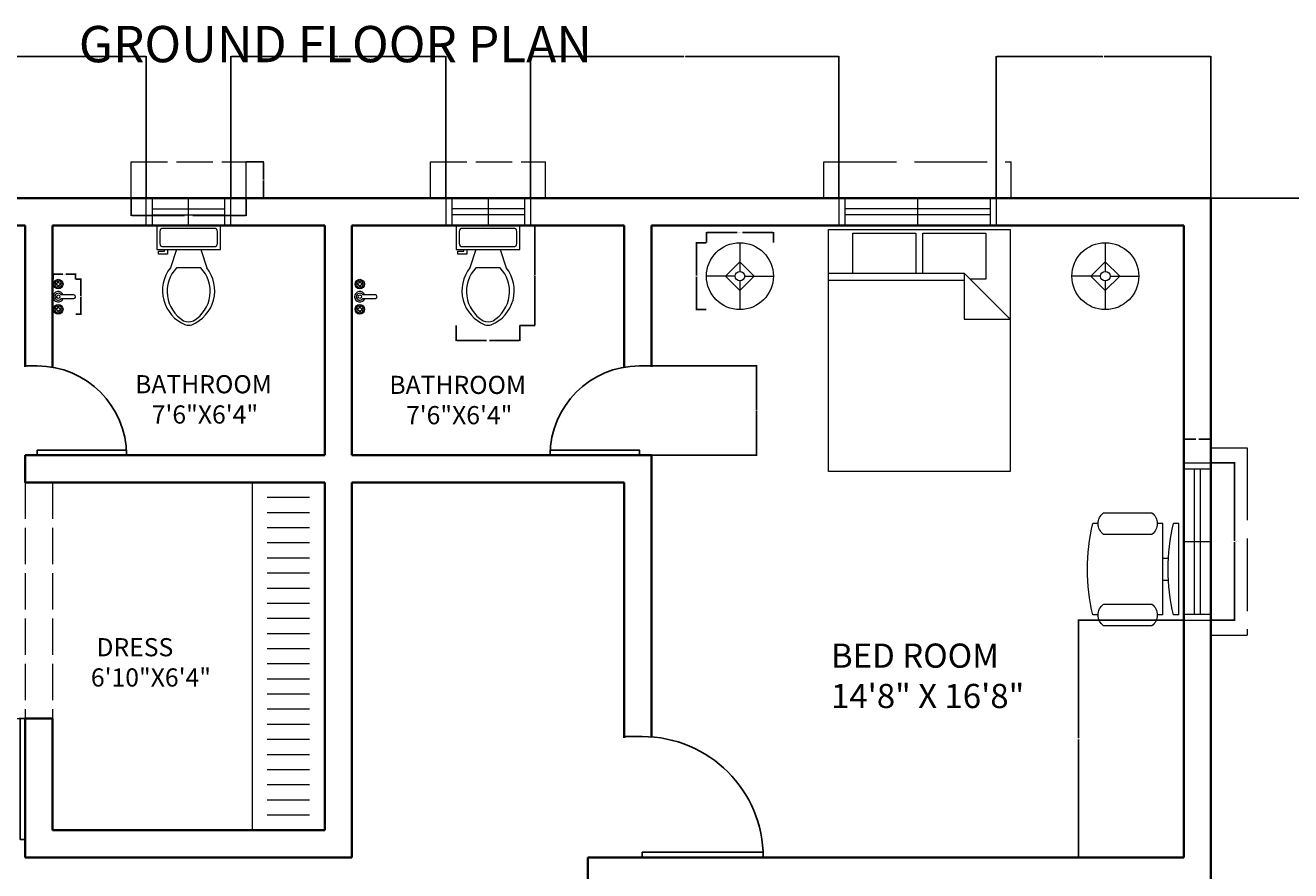
# Model space of a CAD drawing. Units: inches. Extents: x -1138 to 192, y 31 to 760.
# Tile 5 of 6: x -906 to -488, y 478 to 758. Entities that reach past the tile are written whole.
import ezdxf

# ---------------------------------------------------------------- set-up
doc = ezdxf.new("R2010")
doc.units = ezdxf.units.IN
doc.header["$MEASUREMENT"] = 0
doc.linetypes.add('ACAD_ISO02W100', pattern=[15, 12, -3])
for name, color, linetype, lineweight in [('A-ANNO-DIMS', 2, 'Continuous', 18), ('A-ANNO-TEXT', 7, 'Continuous', 25), ('A-AREA-IDEN', 7, 'Continuous', 18), ('A-DOOR', 3, 'Continuous', 25), ('A-FLOR-CASE', 32, 'Continuous', 18), ('A-FLOR-FIXT', 9, 'Continuous', 18), ('A-FURN', 8, 'Continuous', 18), ('A-GLAZ', 4, 'Continuous', 20), ('A-GLAZ-OVHD', 4, 'ACAD_ISO02W100', 13), ('A-WALL', 7, 'Continuous', 35), ('A-WALL-HIDN', 8, 'ACAD_ISO02W100', 18)]:
    doc.layers.add(name, color=color, linetype=linetype, lineweight=lineweight)
doc.styles.get("Standard").update_dxf_attribs({"font": 'arial.ttf'})
doc.dimstyles.get("Standard").update_dxf_attribs({"dimtxt": 0.18, "dimasz": 0.18, "dimexe": 0.18, "dimexo": 0.0625, "dimgap": 0.09, "dimtad": 0, "dimtih": 1, "dimtoh": 1, "dimdec": 1, "dimzin": 0, "dimdsep": 46, "dimlunit": 4, "dimtxsty": 'Standard', "dimcen": 0.09, "dimadec": 0, "dimazin": 0, "dimtfac": 1, "dimtdec": 1, "dimtofl": 0, "dimtmove": 0, "dimatfit": 3, "dimfxl": 1, "dimtolj": 1, "dimtzin": 0, "dimarcsym": 0})

# ---------------------------------------------------------------- blocks, each defined once
blk = doc.blocks.new('*U4')
for p, q in [((0, 0), (0, -6)), ((-40, 0), (-40, -6))]:
    blk.add_line(p, q)
blk.add_lwpolyline([(0, 0), (0, 40), (-1.75, 40), (-1.75, 0)], close=True)
blk.add_arc((0, 0), 40, 90, 180)
blk = doc.blocks.new('*U6')
for p, q in [((0, 0), (0, -100)), ((750, 0), (750, -100))]:
    blk.add_line(p, q)
blk.add_lwpolyline([(0, 0), (0, 750), (43.75, 750), (43.75, 0)], close=True)
blk.add_arc((0, 0), 750, 0, 90)
blk = doc.blocks.new('*U7')
for p, q in [((-750, 0), (-750, -100)), ((0, 0), (0, -100))]:
    blk.add_line(p, q)
blk.add_lwpolyline([(0, 0), (0, 750), (-43.75, 750), (-43.75, 0)], close=True)
blk.add_arc((0, 0), 750, 90, 180)
blk = doc.blocks.new('Bed - Queen')
for p, q in [((0, -80.00003), (0, 0)), ((0, 0), (59.99999, 0)), ((59.99999, 0), (59.99999, -80.00003)), ((7.99999, -1.2), (28.79998, -1.2)), ((7.99999, -14.4), (7.99999, -1.2)), ((28.79998, -1.2), (28.79998, -14.4)), ((31.19999, -1.2), (51.99999, -1.2)), ((31.19999, -14.4), (31.19999, -1.2)), ((51.99999, -1.2), (51.99999, -16.4)), ((0, -14.4), (44.8, -14.4)), ((59.99999, -29.6), (44.8, -14.4)), ((44.8, -14.4), (44.8, -29.6)), ((51.99999, -16.4), (46.79936, -16.4)), ((44.8, -16.8), (0, -16.8)), ((44.8, -29.6), (59.99999, -29.6)), ((59.99999, -80.00003), (0, -80.00003))]:
    blk.add_line(p, q)
blk = doc.blocks.new('Lamp - Table')
for p, q in [((0, 7), (0, 1)), ((0, 3), (-3, 0)), ((3, 0), (0, 3)), ((-1, 0), (-7, 0)), ((-3, 0), (0, -3)), ((0, -3), (3, 0)), ((1, 0), (7, 0)), ((0, -1), (0, -7))]:
    blk.add_line(p, q)
for radius in [7, 1]:
    blk.add_circle((0, 0), radius)
blk = doc.blocks.new('Chair - Desk')
for p, q in [((-8.5, 0), (-8.5, -1)), ((-8.5, 0), (8.5, 0)), ((8.5, 0), (8.5, -1)), ((-2, -3), (-2, -1.9355)), ((2, -1.9576), (2, -3)), ((-8.5, -3), (-8.5, -4)), ((-8.5, -3), (8.5, -3)), ((8.5, -3), (8.5, -4)), ((-10.5, -5), (-10.5, -14)), ((-6.5, -14), (-6.5, -5)), ((6.5, -5), (6.5, -14)), ((10.5, -14), (10.5, -5)), ((-8.5, -15), (-8.5, -16)), ((8.5, -15), (8.5, -16))]:
    blk.add_line(p, q)
for centre, radius, start, end in [((0, 34.625), 36.625, 256.5803, 283.4197), ((-8.5, -6.5), 2.5, 36.8699, 143.1301), ((8.5, -6.5), 2.5, 36.8699, 143.1301), ((-8.5, -12.5), 2.5, 216.8699, 323.1301), ((8.5, -12.5), 2.5, 216.8699, 323.1301), ((0, 19.625), 36.625, 256.5803, 283.4197)]:
    blk.add_arc(centre, radius, start, end)
blk = doc.blocks.new('Toilet - top')
for p, q in [((9.5, -6), (9.5, -2)), ((-8, -8.5), (-8, -8)), ((-7, -8), (-7, -9.5)), ((-4, -8), (-6, -14)), ((4, -8), (6, -14)), ((-10, -8.5), (-8, -8.5)), ((-10, -9.5), (-10, -8.5)), ((-7, -9.5), (-10, -9.5)), ((4, -14), (-4, -14))]:
    blk.add_line(p, q)
blk.add_lwpolyline([(10.5, -8), (10.5, 0), (-10.5, 0), (-10.5, -8)], close=True)
for points in [[(-9.5, -2), (-9.5, -6)], [(8.5, -1), (-8.5, -1)], [(-8.5, -7), (8.5, -7)]]:
    blk.add_lwpolyline(points)
for centre, radius, start, end in [((-8.62, -1.88), 0.884, 81.8699, 188.1301), ((8.62, -1.88), 0.884, 351.8699, 98.1301), ((-8.62, -6.12), 0.884, 171.8699, 278.1301), ((8.62, -6.12), 0.884, 261.8699, 8.1301), ((3.52, -21.58), 12.17, 141.4691, 247.9714), ((4.2, -21.82), 11.33, 136.3677, 238.9468), ((-3.52, -21.58), 12.17, 292.0284, 38.5307), ((-4.2, -21.82), 11.33, 301.053, 43.6321), ((0, -27.88), 4, 245.7318, 294.2682), ((0, -29), 4, 254.8605, 285.1395)]:
    blk.add_arc(centre, radius, start, end)
blk = doc.blocks.new('Faucet - Bathroom top')
for p, q in [((-4.107, 0.125), (-4.375, 0.125)), ((-3.75, 0.4788), (-3.75, 0.75)), ((-3.5, 0.482), (-3.5, 0.75)), ((-3.1461, 0.125), (-2.875, 0.125)), ((3.143, 0.125), (2.875, 0.125)), ((3.5, 0.4788), (3.5, 0.75)), ((3.75, 0.482), (3.75, 0.75)), ((4.1039, 0.125), (4.375, 0.125)), ((-4.1039, -0.125), (-4.375, -0.125)), ((-3.75, -0.4821), (-3.75, -0.75)), ((-3.5, -0.4789), (-3.5, -0.75)), ((-3.143, -0.125), (-2.875, -0.125)), ((-0.5, -0.8639), (-0.5, -4.5)), ((0.5, -4.5), (0.5, -0.8631)), ((3.1461, -0.125), (2.875, -0.125)), ((3.5, -0.4821), (3.5, -0.75)), ((3.75, -0.4789), (3.75, -0.75)), ((4.107, -0.125), (4.375, -0.125))]:
    blk.add_line(p, q)
for centre, radius in [((-3.625, 0), 1.375), ((-4.625, 0), 0.2795), ((-3.625, 0), 0.5), ((-3.625, 1), 0.2795), ((-2.625, 0), 0.2795), ((0, 0), 0.5), ((3.625, 0), 1.375), ((2.625, 0), 0.2795), ((3.625, 0), 0.5), ((3.625, 1), 0.2795), ((4.625, 0), 0.2795), ((-3.625, -1), 0.2795), ((3.625, -1), 0.2795)]:
    blk.add_circle(centre, radius)
for centre, radius, start, end in [((-3.625, 0), 1, 105.2407, 164.2093), ((-3.625, 0), 1, 16.44125, 74.07887), ((0, 0), 1.5, 289.6514, 250.3603), ((0, 0), 1, 300.3431, 239.7554), ((3.625, 0), 1, 106.12, 164.0884), ((3.625, 0), 1, 16.23422, 73.90469), ((-3.625, 0), 1, 196.2342, 253.9047), ((-3.625, 0), 1, 286.12, 344.0884), ((3.625, 0), 1, 196.4413, 254.0789), ((3.625, 0), 1, 285.2407, 344.2093), ((0, -4.5), 0.5, 180, 0)]:
    blk.add_arc(centre, radius, start, end)
blk = doc.blocks.new('WINDOW-48IN')
for p, q in [((0, 0), (0, 9)), ((2, 0), (2, 9)), ((26, 0), (26, 9)), ((50, 0), (50, 9)), ((52, 0), (52, 9)), ((2, 5.5), (50, 5.5)), ((2, 3.5), (50, 3.5))]:
    blk.add_line(p, q)
blk = doc.blocks.new('WINDOW-24IN')
for p, q in [((0, 0), (0, 9)), ((2, 0), (2, 9)), ((14, 0), (14, 9)), ((26, 0), (26, 9)), ((28, 0), (28, 9)), ((2, 5.5), (26, 5.5)), ((2, 3.5), (26, 3.5))]:
    blk.add_line(p, q)
blk = doc.blocks.new('WINDOW-PROJECTION-62IN')
at = {"ltscale": 2}
for p, q in [((0, 0), (0, 12)), ((0, 12), (62, 12)), ((62, 0), (62, 12)), ((5, 0), (0, 0)), ((57, 0), (62, 0))]:
    blk.add_line(p, q, dxfattribs=at)
blk = doc.blocks.new('WINDOW-PROJECTION-38IN')
for p, q in [((0, 0), (0, 12)), ((0, 12), (38, 12)), ((38, 0), (38, 12)), ((5, 0), (0, 0)), ((33, 0), (38, 0))]:
    blk.add_line(p, q)
blk = doc.blocks.new('*D45')
at = {"layer": 'A-ANNO-DIMS', "color": 0, "lineweight": -2, "transparency": 16777216}
for p, q in [((-514.07, 613.31), (-506.15, 613.31)), ((-506.33, 613.13), (-506.33, 587.5)), ((-506.33, 561.49), (-506.33, 587.13)), ((-514.07, 561.31), (-506.15, 561.31))]:
    blk.add_line(p, q, dxfattribs=at)
at = {"layer": 'A-ANNO-DIMS', "color": 0, "transparency": 16777216}
for points in [[(-506.36, 613.13), (-506.3, 613.13), (-506.33, 613.31)], [(-506.36, 561.49), (-506.3, 561.49), (-506.33, 561.31)]]:
    blk.add_solid(points, dxfattribs=at)
at = {"layer": 'Defpoints', "color": 0, "transparency": 16777216}
for p in [(-514.13, 613.31), (-514.13, 561.31), (-506.33, 561.31)]:
    blk.add_point(p, dxfattribs=at)
at = {"layer": 'A-ANNO-DIMS', "color": 0, "transparency": 16777216, "insert": (-506.33, 587.31), "char_height": 0.18, "attachment_point": 5}
blk.add_mtext('\\A1;WINDOW 52 TYP.', dxfattribs=at)
blk = doc.blocks.new('*D46')
at = {"layer": 'A-ANNO-DIMS', "color": 0, "lineweight": -2, "transparency": 16777216}
for p, q in [((-523.13, 613.38), (-523.13, 621.29)), ((-522.95, 621.11), (-519.09, 621.11)), ((-514.31, 621.11), (-518.17, 621.11)), ((-514.13, 613.38), (-514.13, 621.29))]:
    blk.add_line(p, q, dxfattribs=at)
at = {"layer": 'A-ANNO-DIMS', "color": 0, "transparency": 16777216}
for points in [[(-522.95, 621.14), (-522.95, 621.08), (-523.13, 621.11)], [(-514.31, 621.14), (-514.31, 621.08), (-514.13, 621.11)]]:
    blk.add_solid(points, dxfattribs=at)
at = {"layer": 'Defpoints', "color": 0, "transparency": 16777216}
for p in [(-514.13, 621.11), (-523.13, 613.31), (-514.13, 613.31)]:
    blk.add_point(p, dxfattribs=at)
at = {"layer": 'A-ANNO-DIMS', "color": 0, "transparency": 16777216, "insert": (-518.63, 621.11), "char_height": 0.18, "attachment_point": 5}
blk.add_mtext('\\A1;9 TYP.', dxfattribs=at)
blk = doc.blocks.new('*D51')
at = {"layer": 'A-ANNO-DIMS', "color": 0, "lineweight": -2, "transparency": 16777216}
for p, q in [((-871.13, 700.75), (-871.13, 694.93)), ((-833.13, 700.75), (-833.13, 694.93)), ((-870.95, 695.11), (-853.5, 695.11)), ((-833.31, 695.11), (-850.76, 695.11))]:
    blk.add_line(p, q, dxfattribs=at)
at = {"layer": 'A-ANNO-DIMS', "color": 0, "transparency": 16777216}
for points in [[(-870.95, 695.14), (-870.95, 695.08), (-871.13, 695.11)], [(-833.31, 695.14), (-833.31, 695.08), (-833.13, 695.11)]]:
    blk.add_solid(points, dxfattribs=at)
at = {"layer": 'Defpoints', "color": 0, "transparency": 16777216}
for p in [(-871.13, 700.81), (-833.13, 700.81), (-833.13, 695.11)]:
    blk.add_point(p, dxfattribs=at)
at = {"layer": 'A-ANNO-DIMS', "color": 0, "transparency": 16777216, "insert": (-852.13, 695.11), "char_height": 0.18, "attachment_point": 5}
blk.add_mtext('\\A1;PROJECTION 38 TYP.', dxfattribs=at)
blk = doc.blocks.new('*D52')
at = {"layer": 'A-ANNO-DIMS', "color": 0, "lineweight": -2, "transparency": 16777216}
for p, q in [((-833.07, 712.81), (-827.25, 712.81)), ((-827.43, 712.63), (-827.43, 706.99)), ((-827.43, 700.99), (-827.43, 706.63)), ((-833.07, 700.81), (-827.25, 700.81))]:
    blk.add_line(p, q, dxfattribs=at)
at = {"layer": 'A-ANNO-DIMS', "color": 0, "transparency": 16777216}
for points in [[(-827.46, 712.63), (-827.4, 712.63), (-827.43, 712.81)], [(-827.46, 700.99), (-827.4, 700.99), (-827.43, 700.81)]]:
    blk.add_solid(points, dxfattribs=at)
at = {"layer": 'Defpoints', "color": 0, "transparency": 16777216}
for p in [(-833.13, 712.81), (-827.43, 712.81), (-833.13, 700.81)]:
    blk.add_point(p, dxfattribs=at)
at = {"layer": 'A-ANNO-DIMS', "color": 0, "transparency": 16777216, "insert": (-827.43, 706.81), "char_height": 0.18, "attachment_point": 5}
blk.add_mtext('\\A1;12 TYP.', dxfattribs=at)
blk = doc.blocks.new('*D53')
at = {"layer": 'A-ANNO-DIMS', "color": 0, "lineweight": -2, "transparency": 16777216}
for p, q in [((-680.93, 686.16), (-680.93, 689.6)), ((-680.75, 689.42), (-670.77, 689.42)), ((-658.98, 689.42), (-668.96, 689.42)), ((-658.8, 686.16), (-658.8, 689.6))]:
    blk.add_line(p, q, dxfattribs=at)
at = {"layer": 'A-ANNO-DIMS', "color": 0, "transparency": 16777216}
for points in [[(-680.75, 689.45), (-680.75, 689.39), (-680.93, 689.42)], [(-658.98, 689.45), (-658.98, 689.39), (-658.8, 689.42)]]:
    blk.add_solid(points, dxfattribs=at)
at = {"layer": 'Defpoints', "color": 0, "transparency": 16777216}
for p in [(-658.8, 689.42), (-680.93, 686.1), (-658.8, 686.1)]:
    blk.add_point(p, dxfattribs=at)
at = {"layer": 'A-ANNO-DIMS', "color": 0, "transparency": 16777216, "insert": (-669.87, 689.42), "char_height": 0.18, "attachment_point": 5}
blk.add_mtext('\\A1;LAMP 22 TYP.', dxfattribs=at)
blk = doc.blocks.new('*D54')
at = {"layer": 'A-ANNO-DIMS', "color": 0, "lineweight": -2, "transparency": 16777216}
for p, q in [((-681, 686.1), (-684.43, 686.1)), ((-684.25, 685.92), (-684.25, 675.21)), ((-684.25, 664.14), (-684.25, 674.85)), ((-681, 663.96), (-684.43, 663.96))]:
    blk.add_line(p, q, dxfattribs=at)
at = {"layer": 'A-ANNO-DIMS', "color": 0, "transparency": 16777216}
for points in [[(-684.28, 685.92), (-684.22, 685.92), (-684.25, 686.1)], [(-684.28, 664.14), (-684.22, 664.14), (-684.25, 663.96)]]:
    blk.add_solid(points, dxfattribs=at)
at = {"layer": 'Defpoints', "color": 0, "transparency": 16777216}
for p in [(-684.25, 686.1), (-680.93, 686.1), (-680.93, 663.96)]:
    blk.add_point(p, dxfattribs=at)
at = {"layer": 'A-ANNO-DIMS', "color": 0, "transparency": 16777216, "insert": (-684.25, 675.03), "char_height": 0.18, "attachment_point": 5}
blk.add_mtext('\\A1;22 TYP.', dxfattribs=at)
blk = doc.blocks.new('*D65')
at = {"layer": 'A-ANNO-DIMS', "color": 0, "lineweight": -2, "transparency": 16777216}
for p, q in [((-742.57, 691.81), (-737.5, 691.81)), ((-737.68, 691.63), (-737.68, 675.47)), ((-737.68, 658.95), (-737.68, 675.11)), ((-742.57, 658.77), (-737.5, 658.77))]:
    blk.add_line(p, q, dxfattribs=at)
at = {"layer": 'A-ANNO-DIMS', "color": 0, "transparency": 16777216}
for points in [[(-737.71, 691.63), (-737.65, 691.63), (-737.68, 691.81)], [(-737.71, 658.95), (-737.65, 658.95), (-737.68, 658.77)]]:
    blk.add_solid(points, dxfattribs=at)
at = {"layer": 'Defpoints', "color": 0, "transparency": 16777216}
for p in [(-742.63, 691.81), (-737.68, 691.81), (-742.63, 658.77)]:
    blk.add_point(p, dxfattribs=at)
at = {"layer": 'A-ANNO-DIMS', "color": 0, "transparency": 16777216, "insert": (-737.68, 675.29), "char_height": 0.18, "attachment_point": 5}
blk.add_mtext('\\A1;WC 33 TYP.', dxfattribs=at)
blk = doc.blocks.new('*D66')
at = {"layer": 'A-ANNO-DIMS', "color": 0, "lineweight": -2, "transparency": 16777216}
for p, q in [((-763.63, 658.7), (-763.63, 653.63)), ((-742.63, 658.7), (-742.63, 653.63)), ((-763.45, 653.81), (-753.66, 653.81)), ((-742.81, 653.81), (-752.6, 653.81))]:
    blk.add_line(p, q, dxfattribs=at)
at = {"layer": 'A-ANNO-DIMS', "color": 0, "transparency": 16777216}
for points in [[(-763.45, 653.84), (-763.45, 653.78), (-763.63, 653.81)], [(-742.81, 653.84), (-742.81, 653.78), (-742.63, 653.81)]]:
    blk.add_solid(points, dxfattribs=at)
at = {"layer": 'Defpoints', "color": 0, "transparency": 16777216}
for p in [(-763.63, 658.77), (-742.63, 658.77), (-742.63, 653.81)]:
    blk.add_point(p, dxfattribs=at)
at = {"layer": 'A-ANNO-DIMS', "color": 0, "transparency": 16777216, "insert": (-753.13, 653.81), "char_height": 0.18, "attachment_point": 5}
blk.add_mtext('\\A1;21 TYP.', dxfattribs=at)
blk = doc.blocks.new('*D67')
at = {"layer": 'A-ANNO-DIMS', "color": 0, "lineweight": -2, "transparency": 16777216}
for p, q in [((-889.43, 673.99), (-887.59, 673.99)), ((-887.77, 673.81), (-887.77, 668.43)), ((-887.77, 662.68), (-887.77, 668.06)), ((-889.43, 662.5), (-887.59, 662.5))]:
    blk.add_line(p, q, dxfattribs=at)
at = {"layer": 'A-ANNO-DIMS', "color": 0, "transparency": 16777216}
for points in [[(-887.8, 673.81), (-887.74, 673.81), (-887.77, 673.99)], [(-887.8, 662.68), (-887.74, 662.68), (-887.77, 662.5)]]:
    blk.add_solid(points, dxfattribs=at)
at = {"layer": 'Defpoints', "color": 0, "transparency": 16777216}
for p in [(-889.49, 673.99), (-887.77, 673.99), (-889.49, 662.5)]:
    blk.add_point(p, dxfattribs=at)
at = {"layer": 'A-ANNO-DIMS', "color": 0, "transparency": 16777216, "insert": (-887.77, 668.24), "char_height": 0.18, "attachment_point": 5}
blk.add_mtext('\\A1;FAUCET 11 TYP.', dxfattribs=at)
blk = doc.blocks.new('*D68')
at = {"layer": 'A-ANNO-DIMS', "color": 0, "lineweight": -2, "transparency": 16777216}
for p, q in [((-896.96, 674.05), (-896.96, 675.89)), ((-896.78, 675.71), (-893.68, 675.71)), ((-889.67, 675.71), (-892.77, 675.71)), ((-889.49, 674.05), (-889.49, 675.89))]:
    blk.add_line(p, q, dxfattribs=at)
at = {"layer": 'A-ANNO-DIMS', "color": 0, "transparency": 16777216}
for points in [[(-896.78, 675.74), (-896.78, 675.68), (-896.96, 675.71)], [(-889.67, 675.74), (-889.67, 675.68), (-889.49, 675.71)]]:
    blk.add_solid(points, dxfattribs=at)
at = {"layer": 'Defpoints', "color": 0, "transparency": 16777216}
for p in [(-896.96, 675.71), (-896.96, 673.99), (-889.49, 673.99)]:
    blk.add_point(p, dxfattribs=at)
at = {"layer": 'A-ANNO-DIMS', "color": 0, "transparency": 16777216, "insert": (-893.23, 675.71), "char_height": 0.18, "attachment_point": 5}
blk.add_mtext('\\A1;7 TYP.', dxfattribs=at)
blk = doc.blocks.new('*D86')
at = {"layer": 'A-ANNO-DIMS', "color": 0, "lineweight": -2, "transparency": 16777216}
for p, q in [((-514.07, 700.81), (-467.14, 700.81)), ((-467.32, 700.63), (-467.32, 389.49)), ((-467.32, 77.99), (-467.32, 389.13)), ((-514.07, 77.81), (-467.14, 77.81))]:
    blk.add_line(p, q, dxfattribs=at)
at = {"layer": 'A-ANNO-DIMS', "color": 0, "transparency": 16777216}
for points in [[(-467.35, 700.63), (-467.29, 700.63), (-467.32, 700.81)], [(-467.35, 77.99), (-467.29, 77.99), (-467.32, 77.81)]]:
    blk.add_solid(points, dxfattribs=at)
at = {"layer": 'Defpoints', "color": 0, "transparency": 16777216}
for p in [(-514.13, 700.81), (-467.32, 700.81), (-514.13, 77.81)]:
    blk.add_point(p, dxfattribs=at)
at = {"layer": 'A-ANNO-DIMS', "color": 0, "transparency": 16777216, "insert": (-467.32, 389.31), "char_height": 0.18, "attachment_point": 5}
blk.add_mtext('\\A1;623', dxfattribs=at)
blk = doc.blocks.new('*D88')
at = {"layer": 'A-ANNO-DIMS', "color": 0, "lineweight": -2, "transparency": 16777216}
for p, q in [((-968.13, 700.88), (-968.13, 747.81)), ((-967.95, 747.63), (-917.41, 747.63)), ((-866.31, 747.63), (-916.85, 747.63)), ((-866.13, 700.88), (-866.13, 747.81))]:
    blk.add_line(p, q, dxfattribs=at)
at = {"layer": 'A-ANNO-DIMS', "color": 0, "transparency": 16777216}
for points in [[(-967.95, 747.66), (-967.95, 747.6), (-968.13, 747.63)], [(-866.31, 747.66), (-866.31, 747.6), (-866.13, 747.63)]]:
    blk.add_solid(points, dxfattribs=at)
at = {"layer": 'Defpoints', "color": 0, "transparency": 16777216}
for p in [(-866.13, 747.63), (-968.13, 700.81), (-866.13, 700.81)]:
    blk.add_point(p, dxfattribs=at)
at = {"layer": 'A-ANNO-DIMS', "color": 0, "transparency": 16777216, "insert": (-917.13, 747.63), "char_height": 0.18, "attachment_point": 5}
blk.add_mtext('\\A1;102', dxfattribs=at)
blk = doc.blocks.new('*D89')
at = {"layer": 'A-ANNO-DIMS', "color": 0, "lineweight": -2, "transparency": 16777216}
for p, q in [((-838.13, 700.88), (-838.13, 747.81)), ((-837.95, 747.63), (-802.83, 747.63)), ((-767.31, 747.63), (-802.43, 747.63)), ((-767.13, 700.88), (-767.13, 747.81))]:
    blk.add_line(p, q, dxfattribs=at)
at = {"layer": 'A-ANNO-DIMS', "color": 0, "transparency": 16777216}
for points in [[(-837.95, 747.66), (-837.95, 747.6), (-838.13, 747.63)], [(-767.31, 747.66), (-767.31, 747.6), (-767.13, 747.63)]]:
    blk.add_solid(points, dxfattribs=at)
at = {"layer": 'Defpoints', "color": 0, "transparency": 16777216}
for p in [(-767.13, 747.63), (-838.13, 700.81), (-767.13, 700.81)]:
    blk.add_point(p, dxfattribs=at)
at = {"layer": 'A-ANNO-DIMS', "color": 0, "transparency": 16777216, "insert": (-802.63, 747.63), "char_height": 0.18, "attachment_point": 5}
blk.add_mtext('\\A1;71', dxfattribs=at)
blk = doc.blocks.new('*D90')
at = {"layer": 'A-ANNO-DIMS', "color": 0, "lineweight": -2, "transparency": 16777216}
for p, q in [((-739.13, 700.88), (-739.13, 747.81)), ((-738.95, 747.63), (-688.41, 747.63)), ((-637.31, 747.63), (-687.85, 747.63)), ((-637.13, 700.88), (-637.13, 747.81))]:
    blk.add_line(p, q, dxfattribs=at)
at = {"layer": 'A-ANNO-DIMS', "color": 0, "transparency": 16777216}
for points in [[(-738.95, 747.66), (-738.95, 747.6), (-739.13, 747.63)], [(-637.31, 747.66), (-637.31, 747.6), (-637.13, 747.63)]]:
    blk.add_solid(points, dxfattribs=at)
at = {"layer": 'Defpoints', "color": 0, "transparency": 16777216}
for p in [(-637.13, 747.63), (-739.13, 700.81), (-637.13, 700.81)]:
    blk.add_point(p, dxfattribs=at)
at = {"layer": 'A-ANNO-DIMS', "color": 0, "transparency": 16777216, "insert": (-688.13, 747.63), "char_height": 0.18, "attachment_point": 5}
blk.add_mtext('\\A1;102', dxfattribs=at)
blk = doc.blocks.new('*D91')
at = {"layer": 'A-ANNO-DIMS', "color": 0, "lineweight": -2, "transparency": 16777216}
for p, q in [((-585.13, 700.88), (-585.13, 747.81)), ((-584.95, 747.63), (-549.83, 747.63)), ((-514.31, 747.63), (-549.43, 747.63)), ((-514.13, 700.88), (-514.13, 747.81))]:
    blk.add_line(p, q, dxfattribs=at)
at = {"layer": 'A-ANNO-DIMS', "color": 0, "transparency": 16777216}
for points in [[(-584.95, 747.66), (-584.95, 747.6), (-585.13, 747.63)], [(-514.31, 747.66), (-514.31, 747.6), (-514.13, 747.63)]]:
    blk.add_solid(points, dxfattribs=at)
at = {"layer": 'Defpoints', "color": 0, "transparency": 16777216}
for p in [(-514.13, 747.63), (-585.13, 700.81), (-514.13, 700.81)]:
    blk.add_point(p, dxfattribs=at)
at = {"layer": 'A-ANNO-DIMS', "color": 0, "transparency": 16777216, "insert": (-549.63, 747.63), "char_height": 0.18, "attachment_point": 5}
blk.add_mtext('\\A1;71', dxfattribs=at)
blk = doc.blocks.new('*D95')
at = {"layer": 'A-ANNO-DIMS', "color": 0, "lineweight": -2, "transparency": 16777216}
for p, q in [((-523.2, 561.31), (-558.13, 561.31)), ((-557.95, 561.13), (-557.95, 522.24)), ((-557.95, 482.99), (-557.95, 521.88)), ((-523.2, 482.81), (-558.13, 482.81))]:
    blk.add_line(p, q, dxfattribs=at)
at = {"layer": 'A-ANNO-DIMS', "color": 0, "transparency": 16777216}
for points in [[(-557.98, 561.13), (-557.92, 561.13), (-557.95, 561.31)], [(-557.98, 482.99), (-557.92, 482.99), (-557.95, 482.81)]]:
    blk.add_solid(points, dxfattribs=at)
at = {"layer": 'Defpoints', "color": 0, "transparency": 16777216}
for p in [(-557.95, 561.31), (-523.13, 561.31), (-523.13, 482.81)]:
    blk.add_point(p, dxfattribs=at)
at = {"layer": 'A-ANNO-DIMS', "color": 0, "transparency": 16777216, "insert": (-557.95, 522.06), "char_height": 0.18, "attachment_point": 5}
blk.add_mtext('\\A1;78.5', dxfattribs=at)
blk = doc.blocks.new('*D100')
at = {"layer": 'A-ANNO-DIMS', "color": 0, "lineweight": -2, "transparency": 16777216}
for p, q in [((-699.07, 645.34), (-664.14, 645.34)), ((-664.32, 645.16), (-664.32, 630.76)), ((-664.32, 615.99), (-664.32, 630.39)), ((-699.07, 615.81), (-664.14, 615.81))]:
    blk.add_line(p, q, dxfattribs=at)
at = {"layer": 'A-ANNO-DIMS', "color": 0, "transparency": 16777216}
for points in [[(-664.35, 645.16), (-664.29, 645.16), (-664.32, 645.34)], [(-664.35, 615.99), (-664.29, 615.99), (-664.32, 615.81)]]:
    blk.add_solid(points, dxfattribs=at)
at = {"layer": 'Defpoints', "color": 0, "transparency": 16777216}
for p in [(-699.13, 645.34), (-699.13, 615.81), (-664.32, 615.81)]:
    blk.add_point(p, dxfattribs=at)
at = {"layer": 'A-ANNO-DIMS', "color": 0, "transparency": 16777216, "insert": (-664.32, 630.58), "char_height": 0.18, "attachment_point": 5}
blk.add_mtext('\\A1;29.53', dxfattribs=at)

msp = doc.modelspace()

# ---------------------------------------------------------------- linework, layer by layer
at = {"layer": 'A-FLOR-CASE'}
for p, q in [((-807.133, 606.813), (-831.133, 606.813)), ((-831.133, 606.813), (-831.133, 491.813)), ((-812.133, 601.813), (-826.133, 601.813)), ((-812.133, 596.813), (-826.133, 596.813)), ((-812.133, 591.813), (-826.133, 591.813)), ((-812.133, 586.813), (-826.133, 586.813)), ((-812.133, 581.813), (-826.133, 581.813)), ((-812.133, 576.813), (-826.133, 576.813)), ((-812.133, 571.813), (-826.133, 571.813)), ((-812.133, 566.813), (-826.133, 566.813)), ((-812.133, 561.813), (-826.133, 561.813)), ((-812.133, 556.813), (-826.133, 556.813)), ((-812.133, 551.813), (-826.133, 551.813)), ((-812.133, 546.813), (-826.133, 546.813)), ((-812.133, 541.813), (-826.133, 541.813)), ((-812.133, 536.813), (-826.133, 536.813)), ((-812.133, 531.813), (-826.133, 531.813)), ((-812.133, 526.813), (-826.133, 526.813)), ((-812.133, 521.813), (-826.133, 521.813)), ((-812.133, 516.813), (-826.133, 516.813)), ((-812.133, 511.813), (-826.133, 511.813)), ((-812.133, 506.813), (-826.133, 506.813)), ((-812.133, 501.813), (-826.133, 501.813)), ((-812.133, 496.813), (-826.133, 496.813))]:
    msp.add_line(p, q, dxfattribs=at)
at = {"layer": 'A-WALL'}
for p, q in [((-1091.133, 700.813), (-897.133, 700.813)), ((-897.133, 700.813), (-798.133, 700.813)), ((-798.133, 700.813), (-699.133, 700.813)), ((-699.133, 700.813), (-514.133, 700.813)), ((-514.133, 700.813), (-514.133, 482.813)), ((-1082.133, 691.813), (-906.133, 691.813)), ((-906.133, 691.813), (-906.133, 645.077)), ((-897.133, 691.813), (-897.133, 644.903)), ((-897.133, 691.813), (-807.133, 691.813)), ((-807.133, 691.813), (-807.133, 615.813)), ((-798.133, 691.813), (-798.133, 615.813)), ((-798.133, 691.813), (-708.133, 691.813)), ((-708.133, 691.813), (-708.133, 644.903)), ((-708.133, 691.813), (-708.133, 644.903)), ((-699.133, 691.813), (-699.133, 645.077)), ((-699.133, 691.813), (-523.133, 691.813)), ((-523.133, 691.813), (-523.133, 482.813)), ((-807.133, 615.813), (-906.133, 615.813)), ((-906.133, 615.813), (-906.133, 606.813)), ((-798.133, 615.813), (-699.133, 615.813)), ((-699.133, 615.813), (-699.133, 522.7)), ((-906.133, 606.813), (-807.133, 606.813)), ((-815.133, 606.813), (-897.133, 606.813)), ((-807.133, 606.813), (-807.133, 491.813)), ((-798.133, 606.813), (-708.133, 606.813)), ((-798.133, 606.813), (-798.133, 482.813)), ((-708.133, 606.813), (-708.133, 522.36)), ((-906.133, 528.813), (-897.133, 528.813)), ((-906.133, 528.813), (-906.133, 482.813)), ((-897.133, 528.813), (-897.133, 491.813)), ((-807.133, 491.813), (-897.133, 491.813)), ((-798.133, 482.813), (-906.133, 482.813)), ((-720.133, 362.36), (-720.133, 482.813)), ((-708.133, 482.813), (-720.133, 482.813)), ((-708.133, 482.813), (-720.133, 482.813)), ((-523.133, 482.813), (-708.133, 482.813)), ((-523.133, 482.813), (-699.133, 482.813)), ((-514.133, 482.813), (-514.133, 322.813))]:
    msp.add_line(p, q, dxfattribs=at)
at = {"layer": 'A-WALL-HIDN'}
for p, q in [((-906.133, 606.813), (-906.133, 528.813)), ((-897.133, 606.813), (-897.133, 528.813))]:
    msp.add_line(p, q, dxfattribs=at)

# ---------------------------------------------------------------- block references
at = {"layer": 'A-DOOR', "xscale": 0.0393700787401575, "yscale": 0.0393700787401575, "zscale": 0.0393700787401575}
for name, p, rotation in [('*U7', (-902.196, 615.813), 270), ('*U6', (-703.07, 615.813), 90)]:
    msp.add_blockref(name, p, dxfattribs=dict(at, rotation=rotation))
at = {"layer": 'A-DOOR'}
msp.add_blockref('*U4', (-906.133, 488.813), dxfattribs=at)
at = {"layer": 'A-DOOR', "rotation": 270}
msp.add_blockref('*U4', (-702.133, 482.813), dxfattribs=at)
at = {"layer": 'A-FLOR-FIXT'}
for p in [(-852.133, 691.813), (-753.133, 691.813)]:
    msp.add_blockref('Toilet - top', p, dxfattribs=at)
at = {"layer": 'A-FLOR-FIXT', "xscale": 1.149324743471979, "yscale": 1.149324743471979, "zscale": 1.149324743471979, "rotation": 90}
for p in [(-895.237, 668.243), (-795.541, 668.243)]:
    msp.add_blockref('Faucet - Bathroom top', p, dxfattribs=at)
at = {"layer": 'A-FURN'}
msp.add_blockref('Bed - Queen', (-640.529, 690.45), dxfattribs=at)
at = {"layer": 'A-FURN', "xscale": 1.581140411223051, "yscale": 1.581140411223051, "zscale": 1.581140411223051}
for p in [(-669.865, 675.031), (-549.035, 675.031)]:
    msp.add_blockref('Lamp - Table', p, dxfattribs=at)
at = {"layer": 'A-FURN', "xscale": -1.776798148379839, "yscale": 1.776798148379839, "zscale": 1.776798148379839, "rotation": 270}
msp.add_blockref('Chair - Desk', (-524.744, 578.105), dxfattribs=at)
at = {"layer": 'A-GLAZ'}
msp.add_blockref('WINDOW-24IN', (-866.133, 691.813), dxfattribs=at)
for name, p, rotation in [('WINDOW-24IN', (-739.133, 700.813), 180), ('WINDOW-48IN', (-585.133, 700.813), 180), ('WINDOW-48IN', (-523.133, 613.313), 270.0000000000002)]:
    msp.add_blockref(name, p, dxfattribs=dict(at, rotation=rotation))
at = {"layer": 'A-GLAZ-OVHD'}
for name, p in [('WINDOW-PROJECTION-38IN', (-871.133, 700.813)), ('WINDOW-PROJECTION-38IN', (-772.133, 700.813)), ('WINDOW-PROJECTION-62IN', (-642.133, 700.813))]:
    msp.add_blockref(name, p, dxfattribs=at)
at = {"layer": 'A-GLAZ-OVHD', "rotation": 269.9999999999997}
msp.add_blockref('WINDOW-PROJECTION-62IN', (-514.133, 618.313), dxfattribs=at)

# ---------------------------------------------------------------- texts
at = {"layer": 'A-ANNO-TEXT'}
msp.add_text('GROUND FLOOR PLAN', height=12, dxfattribs=at).set_placement((-888.428, 745.758))
at = {"layer": 'A-AREA-IDEN', "attachment_point": 1}
for s, insert, char_height in [('BATHROOM\\P   7\'6"X6\'4"', (-869.828, 642.298), 6), ('BATHROOM\\P   7\'6"X6\'4"', (-785.767, 642.079), 6), (' DRESS\\P6\'10"X6\'4"', (-884.453, 555.35), 6), ('BED ROOM\\P14\'8" X 16\'8"', (-639.738, 553.561), 8)]:
    msp.add_mtext_dynamic_manual_height_columns(s, width=126.58932, gutter_width=1, heights=[0], dxfattribs=dict(at, insert=insert, char_height=char_height))

# ---------------------------------------------------------------- dimensions: what is measured, and where the dimension line sits
at = {"layer": 'A-ANNO-DIMS'}
for base, p1, p2, picture, middle in [((-866.133, 747.628), (-968.133, 700.813), (-866.133, 700.813), '*D88', (-917.133, 747.628)), ((-767.133, 747.628), (-838.133, 700.813), (-767.133, 700.813), '*D89', (-802.633, 747.628)), ((-637.133, 747.628), (-739.133, 700.813), (-637.133, 700.813), '*D90', (-688.133, 747.628)), ((-514.133, 747.628), (-585.133, 700.813), (-514.133, 700.813), '*D91', (-549.633, 747.628))]:
    dim = msp.add_linear_dim(base=base, p1=p1, p2=p2, dimstyle='Standard', override={"dimdec": 0, "dimlfac": 1, "dimrnd": 0, "dimzin": 0, "dimdsep": 46, "dimlunit": 2}, dxfattribs=at)
    dim.commit()
    dim.dimension.update_dxf_attribs({"geometry": picture, "text_midpoint": middle})
for base, p1, p2, angle, text, picture, middle in [((-827.433, 712.813), (-833.133, 700.813), (-833.133, 712.813), 90, '<> TYP.', '*D52', (-827.433, 706.813)), ((-737.676, 691.813), (-742.633, 658.767), (-742.633, 691.813), 90, 'WC <> TYP.', '*D65', (-737.676, 675.29)), ((-684.253, 686.099), (-680.933, 663.963), (-680.933, 686.099), 90, '<> TYP.', '*D54', (-684.253, 675.031)), ((-896.961, 675.714), (-889.491, 673.99), (-896.961, 673.99), 180, '<> TYP.', '*D68', (-893.226, 675.714)), ((-887.767, 673.99), (-889.491, 662.497), (-889.491, 673.99), 90, 'FAUCET <> TYP.', '*D67', (-887.767, 668.243)), ((-506.333, 561.313), (-514.133, 613.313), (-514.133, 561.313), 270, 'WINDOW <> TYP.', '*D45', (-506.333, 587.313))]:
    dim = msp.add_linear_dim(base=base, p1=p1, p2=p2, angle=angle, text=text, dimstyle='Standard', override={"dimdec": 0, "dimlfac": 1, "dimrnd": 0, "dimzin": 0, "dimdsep": 46, "dimlunit": 2}, dxfattribs=at)
    dim.commit()
    dim.dimension.update_dxf_attribs({"geometry": picture, "text_midpoint": middle})
for base, p1, p2, text, picture, middle in [((-833.133, 695.113), (-871.133, 700.813), (-833.133, 700.813), 'PROJECTION <> TYP.', '*D51', (-852.133, 695.113)), ((-658.797, 689.419), (-680.933, 686.099), (-658.797, 686.099), 'LAMP <> TYP.', '*D53', (-669.865, 689.419)), ((-742.633, 653.81), (-763.633, 658.767), (-742.633, 658.767), '<> TYP.', '*D66', (-753.133, 653.81)), ((-514.133, 621.113), (-523.133, 613.313), (-514.133, 613.313), '<> TYP.', '*D46', (-518.633, 621.113))]:
    dim = msp.add_linear_dim(base=base, p1=p1, p2=p2, text=text, dimstyle='Standard', override={"dimdec": 0, "dimlfac": 1, "dimrnd": 0, "dimzin": 0, "dimdsep": 46, "dimlunit": 2}, dxfattribs=at)
    dim.commit()
    dim.dimension.update_dxf_attribs({"geometry": picture, "text_midpoint": middle})
for base, p1, p2, angle, override, picture, middle in [((-467.318, 700.813), (-514.133, 77.813), (-514.133, 700.813), 90, {"dimdec": 0, "dimlfac": 1, "dimrnd": 0, "dimzin": 0, "dimdsep": 46, "dimlunit": 2}, '*D86', (-467.318, 389.313)), ((-664.318, 615.813), (-699.133, 645.341), (-699.133, 615.813), 270, {"dimdec": 2, "dimlfac": 1, "dimrnd": 0, "dimzin": 0, "dimdsep": 46, "dimlunit": 2}, '*D100', (-664.318, 630.577)), ((-557.948, 561.313), (-523.133, 482.813), (-523.133, 561.313), 90, {"dimdec": 1, "dimlfac": 1, "dimrnd": 0, "dimzin": 0, "dimdsep": 46, "dimlunit": 2}, '*D95', (-557.948, 522.063))]:
    dim = msp.add_linear_dim(base=base, p1=p1, p2=p2, angle=angle, dimstyle='Standard', override=override, dxfattribs=at)
    dim.commit()
    dim.dimension.update_dxf_attribs({"geometry": picture, "text_midpoint": middle})

doc.saveas('drawing.dxf')
